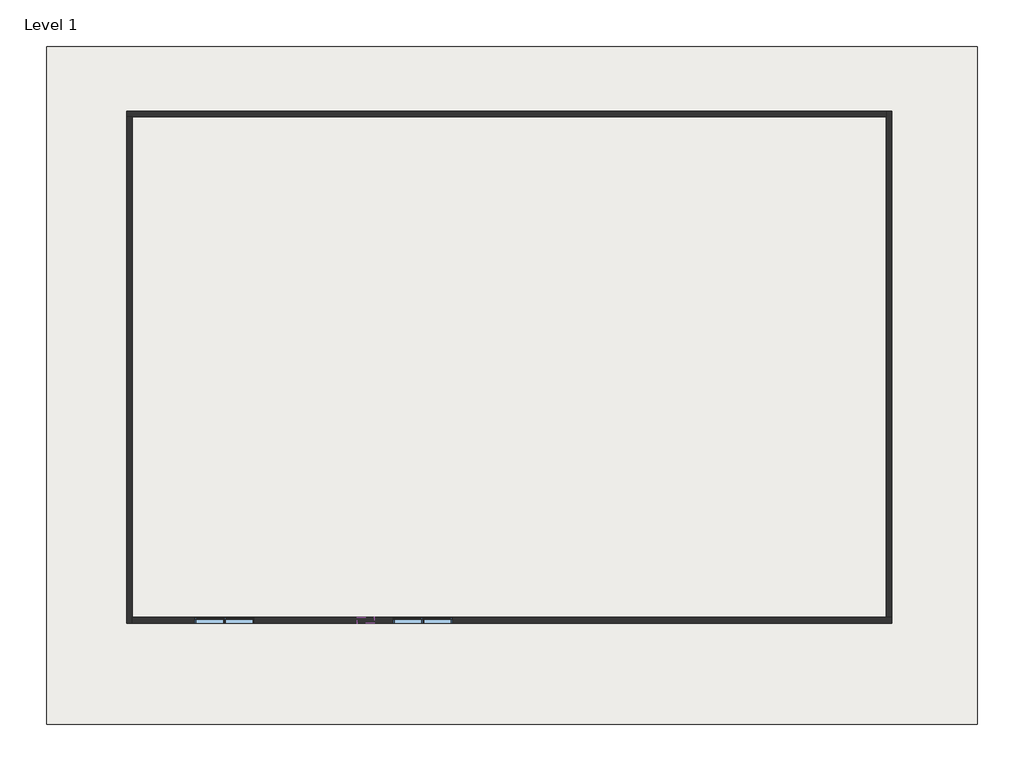
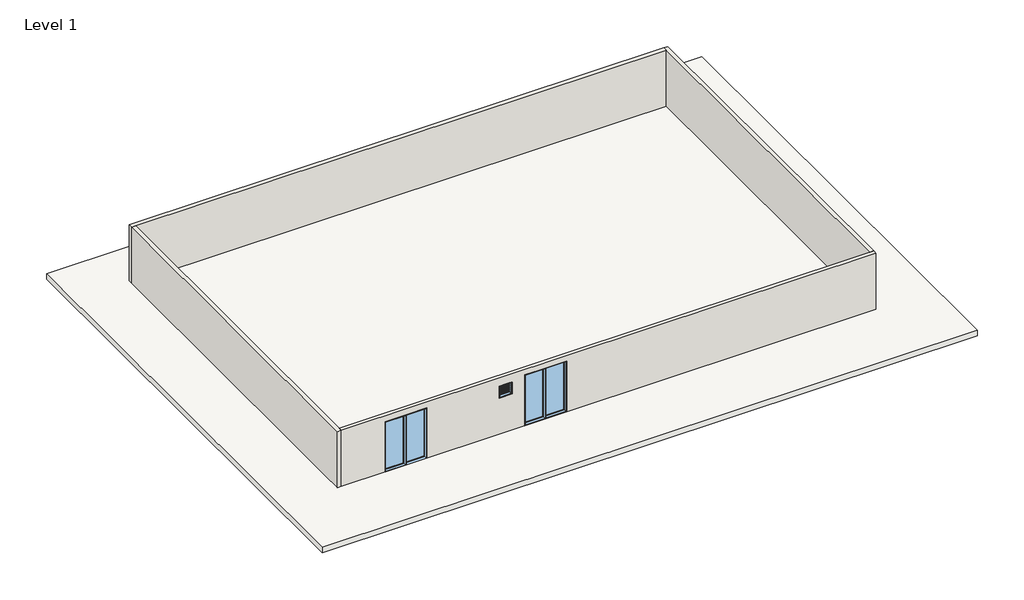
# One storey: 5 windows, 4 walls, 1 slab.
"""IFC4 building model written with IfcOpenShell, lengths in millimetres."""

from ifc_helpers import new_model, si_unit, frame, origin, place, context, project, spatial, polyline, outline, extrude, faceted_brep, transform, mapped, element, save
from components import window_1a213a25, window_0038ecf3

model = new_model("IFC4")

# Units and contexts
model_context = context("Model", 3, world=origin())
ifc_project = project(units=[si_unit("LENGTHUNIT", "METRE", prefix="MILLI")], contexts=[model_context])

# Site, building, storey
site = spatial("IfcSite", under=ifc_project)
building = spatial("IfcBuilding", under=site)
storey = spatial("IfcBuildingStorey", under=building, Name="Level 1", Elevation=0.0)

# Slab
placement = place(None, origin())
element("IfcSlab", 1, ObjectType="Generic - 12\" floor", at=placement, inside=storey, context=model_context, shape_type="SweptSolid", body=[
    extrude(outline(polyline([(12123.2012296, 14036.0758558), (12123.2012296, -10449.5241442), (-21506.3987704, -10449.5241442), (-21506.3987704, 14036.0758558), (12123.2012296, 14036.0758558)])), frame((0.0, 0.0, -304.8), z_axis=(0.0, 0.0, 1.0), x_axis=(1.0, 0.0, 0.0)), (0.0, 0.0, 1.0), 304.8),
])

# Walls
element("IfcWall", 2, ObjectType="Generic - 8\" green", at=placement, inside=storey, context=model_context, shape_type="Brep", body=[
    faceted_brep([(-18610.7987704, 11496.0758558, 0.0), (-18407.5987704, 11496.0758558, 0.0), (8821.2012296, 11496.0758558, 0.0), (8821.2012296, 11496.0758558, 3048.0), (-18407.5987704, 11496.0758558, 3048.0), (-18610.7987704, 11496.0758558, 3048.0), (-18610.7987704, 11699.2758558, 0.0), (-18610.7987704, 11699.2758558, 3048.0), (8821.2012296, 11699.2758558, 3048.0), (8821.2012296, 11699.2758558, 0.0)], [[[0, 1, 2, 3, 4, 5]], [[6, 7, 8, 9]], [[2, 1, 0, 6, 9]], [[5, 4, 3, 8, 7]], [[0, 5, 7, 6]], [[3, 2, 9, 8]]]),
])
element("IfcWall", 3, ObjectType="Generic - 8\" green", at=placement, inside=storey, context=model_context, shape_type="Brep", body=[
    faceted_brep([(-18407.5987704, -6791.9241442, 0.0), (-18407.5987704, -6588.7241442, 0.0), (-18407.5987704, 11496.0758558, 0.0), (-18407.5987704, 11496.0758558, 3048.0), (-18407.5987704, -6588.7241442, 3048.0), (-18407.5987704, -6791.9241442, 3048.0), (-18610.7987704, -6791.9241442, 0.0), (-18610.7987704, -6791.9241442, 3048.0), (-18610.7987704, 11496.0758558, 3048.0), (-18610.7987704, 11496.0758558, 0.0)], [[[0, 1, 2, 3, 4, 5]], [[6, 7, 8, 9]], [[2, 1, 0, 6, 9]], [[0, 5, 7, 6]], [[3, 2, 9, 8]], [[5, 4, 3, 8, 7]]]),
])
element("IfcWall", 4, ObjectType="Generic - 8\" green", at=placement, inside=storey, context=model_context, shape_type="Brep", body=[
    faceted_brep([(9024.4012296, -6588.7241442, 3048.0), (9024.4012296, -6588.7241442, 0.0), (8821.2012296, -6588.7241442, 0.0), (-14013.3987704, -6588.7241442, 0.0), (-14013.3987704, -6588.7241442, 2725.7775861), (-16146.9987704, -6588.7241442, 2725.7775861), (-16146.9987704, -6588.7241442, 0.0), (-18407.5987704, -6588.7241442, 0.0), (-18407.5987704, -6588.7241442, 3048.0), (8821.2012296, -6588.7241442, 3048.0), (-9669.9987704, -6588.7241442, 2590.2004095), (-10279.5987704, -6588.7241442, 2590.2004095), (-10279.5987704, -6588.7241442, 1980.6004095), (-9669.9987704, -6588.7241442, 1980.6004095), (-8984.1987704, -6588.7241442, 7.4818364), (-7917.3987704, -6588.7241442, 7.4818364), (-7917.3987704, -6588.7241442, 10.0444711), (-6850.5987704, -6588.7241442, 10.0444711), (-6850.5987704, -6588.7241442, 2753.2444711), (-7917.3987704, -6588.7241442, 2753.2444711), (-7917.3987704, -6588.7241442, 2750.6818364), (-8984.1987704, -6588.7241442, 2750.6818364), (9024.4012296, -6791.9241442, 0.0), (9024.4012296, -6791.9241442, 3048.0), (-18407.5987704, -6791.9241442, 3048.0), (-18407.5987704, -6791.9241442, 0.0), (-16146.9987704, -6791.9241442, 0.0), (-16146.9987704, -6791.9241442, 2725.7775861), (-14013.3987704, -6791.9241442, 2725.7775861), (-14013.3987704, -6791.9241442, 0.0), (-9669.9987704, -6791.9241442, 2590.2004095), (-9669.9987704, -6791.9241442, 1980.6004095), (-10279.5987704, -6791.9241442, 1980.6004095), (-10279.5987704, -6791.9241442, 2590.2004095), (-7917.3987704, -6791.9241442, 7.4818364), (-8984.1987704, -6791.9241442, 7.4818364), (-8984.1987704, -6791.9241442, 2750.6818364), (-7917.3987704, -6791.9241442, 2750.6818364), (-7917.3987704, -6791.9241442, 2753.2444711), (-6850.5987704, -6791.9241442, 2753.2444711), (-6850.5987704, -6791.9241442, 10.0444711), (-7917.3987704, -6791.9241442, 10.0444711)], [[[0, 1, 2, 3, 4, 5, 6, 7, 8, 9], [10, 11, 12, 13], [14, 15, 16, 17, 18, 19, 20, 21]], [[22, 23, 24, 25, 26, 27, 28, 29], [30, 31, 32, 33], [34, 35, 36, 37, 38, 39, 40, 41]], [[1, 22, 29, 3, 2]], [[25, 7, 6, 26]], [[1, 0, 23, 22]], [[8, 7, 25, 24]], [[0, 9, 8, 24, 23]], [[5, 27, 26, 6]], [[27, 5, 4, 28]], [[28, 4, 3, 29]], [[31, 30, 10, 13]], [[32, 31, 13, 12]], [[33, 32, 12, 11]], [[30, 33, 11, 10]], [[15, 34, 41, 16]], [[35, 34, 15, 14]], [[36, 35, 14, 21]], [[37, 36, 21, 20]], [[39, 18, 17, 40]], [[19, 38, 37, 20]], [[18, 39, 38, 19]], [[40, 17, 16, 41]]]),
])
element("IfcWall", 5, ObjectType="Generic - 8\" green", at=placement, inside=storey, context=model_context, shape_type="Brep", body=[
    faceted_brep([(8821.2012296, 11699.2758558, 0.0), (8821.2012296, 11496.0758558, 0.0), (8821.2012296, -6588.7241442, 0.0), (8821.2012296, -6588.7241442, 3048.0), (8821.2012296, 11496.0758558, 3048.0), (8821.2012296, 11699.2758558, 3048.0), (9024.4012296, 11699.2758558, 0.0), (9024.4012296, 11699.2758558, 3048.0), (9024.4012296, -6588.7241442, 3048.0), (9024.4012296, -6588.7241442, 0.0)], [[[0, 1, 2, 3, 4, 5]], [[6, 7, 8, 9]], [[2, 1, 0, 6, 9]], [[0, 5, 7, 6]], [[3, 2, 9, 8]], [[5, 4, 3, 8, 7]]]),
])

# Windows
window_shape = window_1a213a25(model_context)
element("IfcWindow", 6, ObjectType="Fixed : 36\" x 72\" 2", at=placement, inside=storey, context=model_context, shape_type="MappedRepresentation", body=[
    mapped(window_shape, transform((-15575.4987704, -6690.3241442, -322.2224139), x_axis=(1.0, 0.0, 0.0), y_axis=(0.0, 1.0, 0.0), z_axis=(0.0, 0.0, 1.0))),
])
element("IfcWindow", 7, ObjectType="Fixed : 36\" x 72\" 2", at=placement, inside=storey, context=model_context, shape_type="MappedRepresentation", body=[
    mapped(window_shape, transform((-14508.6987704, -6690.3241442, -322.2224139), x_axis=(1.0, 0.0, 0.0), y_axis=(0.0, 1.0, 0.0), z_axis=(0.0, 0.0, 1.0))),
])
element("IfcWindow", 8, ObjectType="Fixed : 36\" x 72\" 2", at=placement, inside=storey, context=model_context, shape_type="MappedRepresentation", body=[
    mapped(window_shape, transform((-8412.6987704, -6690.3241442, -297.3181636), x_axis=(1.0, 0.0, 0.0), y_axis=(0.0, 1.0, 0.0), z_axis=(0.0, 0.0, 1.0))),
])
element("IfcWindow", 9, ObjectType="Fixed : 36\" x 72\" 2", at=placement, inside=storey, context=model_context, shape_type="MappedRepresentation", body=[
    mapped(window_shape, transform((-7345.8987704, -6690.3241442, -294.7555289), x_axis=(1.0, 0.0, 0.0), y_axis=(0.0, 1.0, 0.0), z_axis=(0.0, 0.0, 1.0))),
])
window_2_shape = window_0038ecf3(model_context)
element("IfcWindow", 10, ObjectType="Louvers with Trim : 24\" x 24\"", at=placement, inside=storey, context=model_context, shape_type="MappedRepresentation", body=[
    mapped(window_2_shape, transform((-9974.7987704, -6683.9741442, 1066.2004095), x_axis=(1.0, 0.0, 0.0), y_axis=(0.0, 1.0, 0.0), z_axis=(0.0, 0.0, 1.0))),
])

save(model, "model.ifc")

# Revit data of these elements
# Type "Generic - 12\" floor"
#   Assembly Code = "B1010"
#   Thickness = 1' - 0"
#   Function = 0
#   Layers, outside or top first: 1' - 0" "Default Floor" (function 1)
# Type "Generic - 8\" green"
#   Assembly Code = "B2010"
#   Width = 0' - 8"
#   Layers, outside or top first: 0' - 8" "Damp-proofing" (function 1)
# Type "Fixed : 36\" x 72\" 2"
#   Type Mark = "29"
#   Construction Type Id = "GSP4R"
#   Assembly Code = "B2020100"
#   Analytic Construction = "1/8 in Pilkington single glazing"
#   Visual Light Transmittance = 0.9
#   Solar Heat Gain Coefficient = 0.78
#   Heat Transfer Coefficient (U) = 3.6886 W/(m²·K)
#   Height = 9' - 0"
#   Default Sill Height = 1' - 0"
#   Width = 3' - 6"
#   Window Inset = 0' - 0 3/4"
#   Glass Pane Material = Glass
#   Sash Material = Iron, Ductile
#   Wall Closure = (empty or 0)
# Type "Louvers with Trim : 24\" x 24\""
#   Type Mark = "27"
#   Construction Type Id = "GSP4R"
#   Assembly Code = "B20"
#   Analytic Construction = "1/8 in Pilkington single glazing"
#   Visual Light Transmittance = 0.9
#   Solar Heat Gain Coefficient = 0.78
#   Heat Transfer Coefficient (U) = 3.6886 W/(m²·K)
#   Default Sill Height = 3' - 0"
#   Trim Projection - Ext. = 0' - 0 1/2"
#   Trim Projection - Int. = 0' - 0 1/2"
#   Trim Width - Exterior = 0' - 1 1/2"
#   Trim Width - Interior = 0' - 1 1/2"
#   Width = 2' - 0"
#   Frame Material = Iron, Ductile
#   Louver Material = Glass
#   Trim Exterior Material = Glass
#   Trim Interior Material = Iron, Ductile
#   Wall Closure = (empty or 0)
# Element 1 (IfcSlab, "Generic - 12\" floor")
#   Height Offset From Level = 0' - 0"
#   Phase Created = New Construction
#   Materials on its faces: "Default Floor"
# Elements 2, 3, 4, 5 (IfcWall, "Generic - 8\" green")
#   Top Offset = 0' - 0"
#   Base Offset = 0' - 0"
#   Unconnected Height = 10' - 0"
#   wall height = 10' - 0"
#   Phase Created = New Construction
#   Base Constraint = Level 1
#   Materials on its faces: "Damp-proofing"
# Element 6 (IfcWindow, "Fixed : 36\" x 72\" 2")
#   Mark = "634"
#   Phase Created = New Construction
#   Materials on its faces: "Iron, Ductile", "Glass"
# Element 7 (IfcWindow, "Fixed : 36\" x 72\" 2")
#   Mark = "635"
#   Phase Created = New Construction
#   Materials on its faces: "Iron, Ductile", "Glass"
# Element 8 (IfcWindow, "Fixed : 36\" x 72\" 2")
#   Mark = "637"
#   Phase Created = New Construction
#   Materials on its faces: "Iron, Ductile", "Glass"
# Element 9 (IfcWindow, "Fixed : 36\" x 72\" 2")
#   Mark = "638"
#   Phase Created = New Construction
#   Materials on its faces: "Iron, Ductile", "Glass"
# Element 10 (IfcWindow, "Louvers with Trim : 24\" x 24\"")
#   Mark = "636"
#   Phase Created = New Construction
#   Materials on its faces: "Glass", "Iron, Ductile"
# Materials
#   "Default Floor": colour RGB 128 128 128, transparency 0, Cost = 0
#   "Damp-proofing": class "Generic", colour RGB 127 127 127, transparency 0, Description = "Damp-proofing", Cost = 0
#   "Glass": class "Glass", colour RGB 0 128 192, transparency 0.75, Description = "Soda Lime Glass", Cost = 0
#   "Iron, Ductile": class "Metal", colour RGB 0 0 0, transparency 0, Description = "Ductile cast iron", Cost = 0
